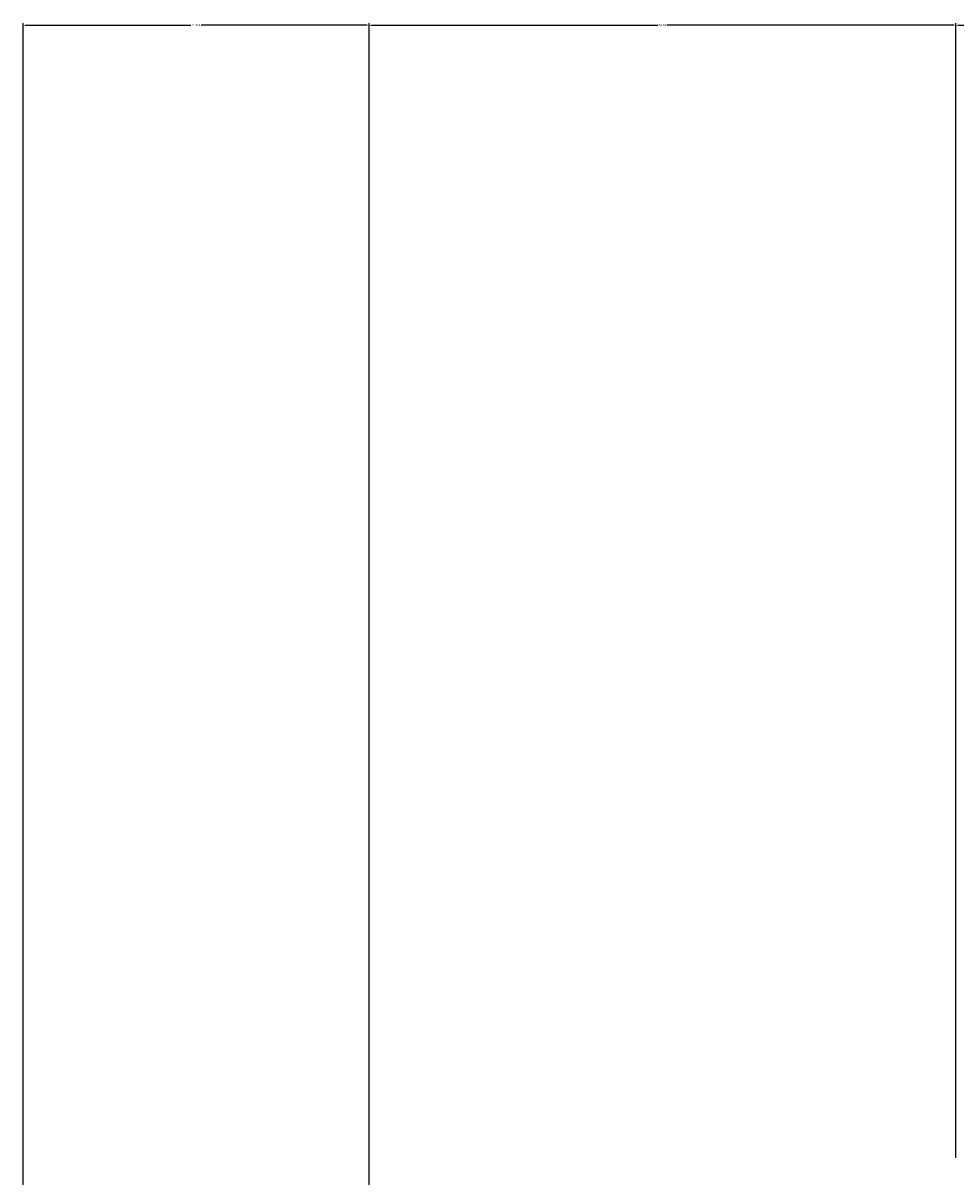
# Model space of a CAD drawing. Units: millimetres. Extents: x 446512 to 447461, y 70395 to 70610.
# Tile 32 of 39: x 447255 to 447340, y 70505 to 70610. Entities that reach past the tile are written whole.
import ezdxf

# ---------------------------------------------------------------- set-up
doc = ezdxf.new("R2010")
doc.units = ezdxf.units.MM
doc.layers.add('A-ANNO-DIMS', color=2, linetype='Continuous', lineweight=18)
doc.styles.get("Standard").update_dxf_attribs({"font": 'arial.ttf'})
doc.dimstyles.get("Standard").update_dxf_attribs({"dimtxt": 0.18, "dimasz": 0.18, "dimexe": 0.18, "dimexo": 0.0625, "dimgap": 0.09, "dimtad": 0, "dimtih": 1, "dimtoh": 1, "dimdec": 4, "dimzin": 0, "dimdsep": 46, "dimtxsty": 'Standard', "dimcen": 0.09, "dimadec": 0, "dimazin": 0, "dimtfac": 1, "dimtdec": 4, "dimtofl": 0, "dimtmove": 0, "dimatfit": 3, "dimfxl": 1, "dimtolj": 1, "dimtzin": 0, "dimarcsym": 0})

# ---------------------------------------------------------------- blocks, each defined once
blk = doc.blocks.new('*D62')
at = {"layer": 'A-ANNO-DIMS', "color": 0, "lineweight": -2, "transparency": 16777216}
for p, q in [((447254.94, 70456.95), (447254.94, 70610.14)), ((447286.51, 70475.94), (447286.51, 70610.14)), ((447255.12, 70609.96), (447270.26, 70609.96)), ((447286.33, 70609.96), (447271.19, 70609.96))]:
    blk.add_line(p, q, dxfattribs=at)
at = {"layer": 'A-ANNO-DIMS', "color": 0, "transparency": 16777216}
for points in [[(447255.12, 70609.99), (447255.12, 70609.93), (447254.94, 70609.96)], [(447286.33, 70609.99), (447286.33, 70609.93), (447286.51, 70609.96)]]:
    blk.add_solid(points, dxfattribs=at)
at = {"layer": 'Defpoints', "color": 0, "transparency": 16777216}
for p in [(447286.51, 70609.96), (447286.51, 70475.88), (447254.94, 70456.89)]:
    blk.add_point(p, dxfattribs=at)
at = {"layer": 'A-ANNO-DIMS', "color": 0, "transparency": 16777216, "insert": (447270.73, 70609.96), "char_height": 0.18, "attachment_point": 5}
blk.add_mtext('\\A1;31.566', dxfattribs=at)
blk = doc.blocks.new('*D63')
at = {"layer": 'A-ANNO-DIMS', "color": 0, "lineweight": -2, "transparency": 16777216}
for p, q in [((447286.51, 70475.94), (447286.51, 70610.14)), ((447340.05, 70506.61), (447340.05, 70610.14)), ((447286.69, 70609.96), (447312.89, 70609.96)), ((447339.87, 70609.96), (447313.67, 70609.96))]:
    blk.add_line(p, q, dxfattribs=at)
at = {"layer": 'A-ANNO-DIMS', "color": 0, "transparency": 16777216}
for points in [[(447286.69, 70609.99), (447286.69, 70609.93), (447286.51, 70609.96)], [(447339.87, 70609.99), (447339.87, 70609.93), (447340.05, 70609.96)]]:
    blk.add_solid(points, dxfattribs=at)
at = {"layer": 'Defpoints', "color": 0, "transparency": 16777216}
for p in [(447340.05, 70609.96), (447340.05, 70506.55), (447286.51, 70475.88)]:
    blk.add_point(p, dxfattribs=at)
at = {"layer": 'A-ANNO-DIMS', "color": 0, "transparency": 16777216, "insert": (447313.28, 70609.96), "char_height": 0.18, "attachment_point": 5}
blk.add_mtext('\\A1;53.54', dxfattribs=at)
blk = doc.blocks.new('*D64')
at = {"layer": 'A-ANNO-DIMS', "color": 0, "lineweight": -2, "transparency": 16777216}
for p, q in [((447340.05, 70506.61), (447340.05, 70610.14)), ((447365.43, 70599.78), (447365.43, 70610.14)), ((447340.23, 70609.96), (447352.27, 70609.96)), ((447365.25, 70609.96), (447353.2, 70609.96))]:
    blk.add_line(p, q, dxfattribs=at)
at = {"layer": 'A-ANNO-DIMS', "color": 0, "transparency": 16777216}
for points in [[(447340.23, 70609.99), (447340.23, 70609.93), (447340.05, 70609.96)], [(447365.25, 70609.99), (447365.25, 70609.93), (447365.43, 70609.96)]]:
    blk.add_solid(points, dxfattribs=at)
at = {"layer": 'Defpoints', "color": 0, "transparency": 16777216}
for p in [(447365.43, 70609.96), (447365.43, 70599.71), (447340.05, 70506.55)]:
    blk.add_point(p, dxfattribs=at)
at = {"layer": 'A-ANNO-DIMS', "color": 0, "transparency": 16777216, "insert": (447352.74, 70609.96), "char_height": 0.18, "attachment_point": 5}
blk.add_mtext('\\A1;25.376', dxfattribs=at)

msp = doc.modelspace()

# ---------------------------------------------------------------- dimensions: what is measured, and where the dimension line sits
at = {"layer": 'A-ANNO-DIMS'}
for base, p1, p2, override, picture, middle in [((447286.5086, 70609.9647), (447254.9427, 70456.89), (447286.5086, 70475.8806), {"dimdec": 3, "dimlfac": 1, "dimrnd": 0, "dimzin": 0, "dimdsep": 46, "dimlunit": 2}, '*D62', (447270.7256, 70609.9647)), ((447340.0494, 70609.9647), (447286.5086, 70475.8806), (447340.0494, 70506.5496), {"dimdec": 2, "dimlfac": 1, "dimrnd": 0, "dimzin": 0, "dimdsep": 46, "dimlunit": 2}, '*D63', (447313.279, 70609.9647)), ((447365.4251, 70609.9647), (447340.0494, 70506.5496), (447365.4251, 70599.7147), {"dimdec": 3, "dimlfac": 1, "dimrnd": 0, "dimzin": 0, "dimdsep": 46, "dimlunit": 2}, '*D64', (447352.7372, 70609.9647))]:
    dim = msp.add_linear_dim(base=base, p1=p1, p2=p2, dimstyle='Standard', override=override, dxfattribs=at)
    dim.commit()
    dim.dimension.update_dxf_attribs({"geometry": picture, "text_midpoint": middle})

doc.saveas('drawing.dxf')
